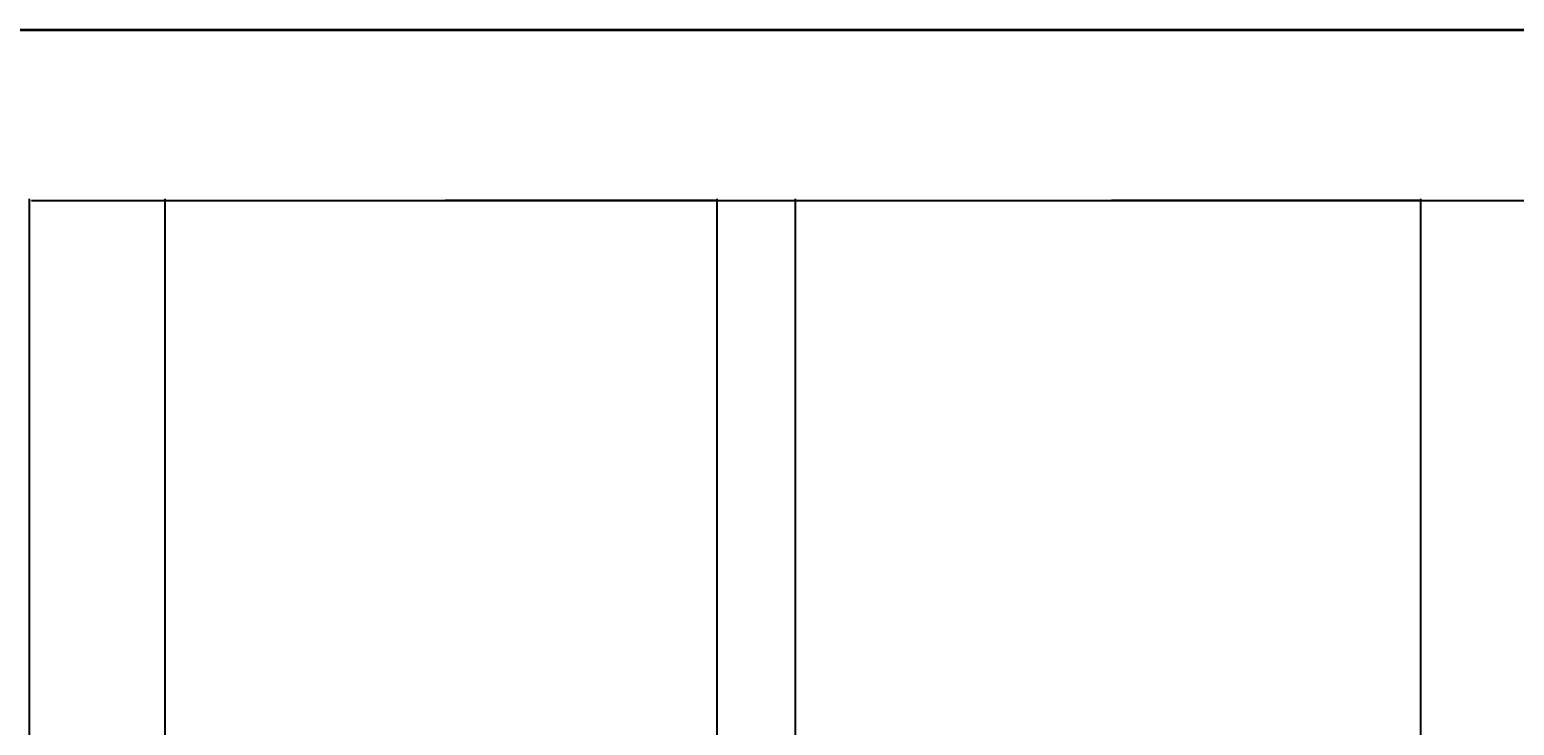
# Model space of a CAD drawing. Units: inches. Extents: x 1088 to 1703, y 668 to 1875.
# Tile 18 of 45: x 1170 to 1319, y 1805 to 1875. Entities that reach past the tile are written whole.
import ezdxf

# ---------------------------------------------------------------- set-up
doc = ezdxf.new("R2010")
doc.units = ezdxf.units.IN
doc.layers.add('A-ANNO-DIMS', color=2, linetype='Continuous', lineweight=18)
doc.layers.add('A-ANNO-TTLB', color=7, linetype='Continuous', lineweight=35)
doc.styles.get("Standard").update_dxf_attribs({"font": 'arial.ttf'})
doc.dimstyles.get("Standard").update_dxf_attribs({"dimtxt": 0.18, "dimasz": 0.18, "dimexe": 0.18, "dimexo": 0.0625, "dimgap": 0.09, "dimtad": 0, "dimtih": 1, "dimtoh": 1, "dimdec": 4, "dimzin": 0, "dimdsep": 46, "dimtxsty": 'Standard', "dimcen": 0.09, "dimadec": 0, "dimazin": 0, "dimtfac": 1, "dimtdec": 4, "dimtofl": 0, "dimtmove": 0, "dimatfit": 3, "dimfxl": 1, "dimtolj": 1, "dimtzin": 0, "dimarcsym": 0})

# ---------------------------------------------------------------- blocks, each defined once
blk = doc.blocks.new('*D28')
at = {"layer": 'A-ANNO-DIMS', "color": 0, "lineweight": -2, "transparency": 16777216}
for p, q in [((1170.34, 1803.62), (1170.34, 1857.79)), ((1170.52, 1857.61), (1408.15, 1857.61)), ((1646.56, 1857.61), (1408.94, 1857.61)), ((1646.74, 1745.55), (1646.74, 1857.79))]:
    blk.add_line(p, q, dxfattribs=at)
at = {"layer": 'A-ANNO-DIMS', "color": 0, "transparency": 16777216}
for points in [[(1170.52, 1857.64), (1170.52, 1857.58), (1170.34, 1857.61)], [(1646.56, 1857.64), (1646.56, 1857.58), (1646.74, 1857.61)]]:
    blk.add_solid(points, dxfattribs=at)
at = {"layer": 'Defpoints', "color": 0, "transparency": 16777216}
for p in [(1646.74, 1857.61), (1170.34, 1803.56), (1646.74, 1745.49)]:
    blk.add_point(p, dxfattribs=at)
at = {"layer": 'A-ANNO-DIMS', "color": 0, "transparency": 16777216, "insert": (1408.54, 1857.61), "char_height": 0.18, "attachment_point": 5}
blk.add_mtext('\\A1;476.4', dxfattribs=at)
blk = doc.blocks.new('*D35')
at = {"layer": 'A-ANNO-DIMS', "color": 0, "lineweight": -2, "transparency": 16777216}
for p, q in [((1183.89, 1448.1), (1183.89, 1857.79)), ((1184.07, 1857.61), (1211.07, 1857.61)), ((1238.86, 1857.61), (1211.86, 1857.61)), ((1239.04, 1448.1), (1239.04, 1857.79))]:
    blk.add_line(p, q, dxfattribs=at)
at = {"layer": 'A-ANNO-DIMS', "color": 0, "transparency": 16777216}
for points in [[(1184.07, 1857.64), (1184.07, 1857.58), (1183.89, 1857.61)], [(1238.86, 1857.64), (1238.86, 1857.58), (1239.04, 1857.61)]]:
    blk.add_solid(points, dxfattribs=at)
at = {"layer": 'Defpoints', "color": 0, "transparency": 16777216}
for p in [(1239.04, 1857.61), (1183.89, 1448.04), (1239.04, 1448.04)]:
    blk.add_point(p, dxfattribs=at)
at = {"layer": 'A-ANNO-DIMS', "color": 0, "transparency": 16777216, "insert": (1211.47, 1857.61), "char_height": 0.18, "attachment_point": 5}
blk.add_mtext('\\A1;55.15', dxfattribs=at)
blk = doc.blocks.new('*D36')
at = {"layer": 'A-ANNO-DIMS', "color": 0, "lineweight": -2, "transparency": 16777216}
for p, q in [((1246.85, 1448.35), (1246.85, 1857.79)), ((1247.03, 1857.61), (1277.78, 1857.61)), ((1309.17, 1857.61), (1278.43, 1857.61)), ((1309.35, 1448.35), (1309.35, 1857.79))]:
    blk.add_line(p, q, dxfattribs=at)
at = {"layer": 'A-ANNO-DIMS', "color": 0, "transparency": 16777216}
for points in [[(1247.03, 1857.64), (1247.03, 1857.58), (1246.85, 1857.61)], [(1309.17, 1857.64), (1309.17, 1857.58), (1309.35, 1857.61)]]:
    blk.add_solid(points, dxfattribs=at)
at = {"layer": 'Defpoints', "color": 0, "transparency": 16777216}
for p in [(1309.35, 1857.61), (1246.85, 1448.29), (1309.35, 1448.29)]:
    blk.add_point(p, dxfattribs=at)
at = {"layer": 'A-ANNO-DIMS', "color": 0, "transparency": 16777216, "insert": (1278.1, 1857.61), "char_height": 0.18, "attachment_point": 5}
blk.add_mtext('\\A1;62.5', dxfattribs=at)

msp = doc.modelspace()

# ---------------------------------------------------------------- linework, layer by layer
at = {"layer": 'A-ANNO-TTLB'}
msp.add_lwpolyline([(1088.369, 1874.677), (1703.181, 1874.677), (1703.181, 667.947), (1088.369, 667.947)], close=True, dxfattribs=at)

# ---------------------------------------------------------------- dimensions: what is measured, and where the dimension line sits
at = {"layer": 'A-ANNO-DIMS'}
for base, p1, p2, override, picture, middle in [((1646.743, 1857.608), (1170.345, 1803.558), (1646.743, 1745.49), {"dimdec": 1, "dimlfac": 1, "dimrnd": 0, "dimzin": 0, "dimdsep": 46, "dimlunit": 2}, '*D28', (1408.544, 1857.608)), ((1239.039, 1857.608), (1183.893, 1448.04), (1239.039, 1448.04), {"dimdec": 2, "dimlfac": 1, "dimrnd": 0, "dimzin": 0, "dimdsep": 46, "dimlunit": 2}, '*D35', (1211.466, 1857.608)), ((1309.352, 1857.608), (1246.852, 1448.287), (1309.352, 1448.287), {"dimdec": 1, "dimlfac": 1, "dimrnd": 0, "dimzin": 0, "dimdsep": 46, "dimlunit": 2}, '*D36', (1278.102, 1857.608))]:
    dim = msp.add_linear_dim(base=base, p1=p1, p2=p2, dimstyle='Standard', override=override, dxfattribs=at)
    dim.commit()
    dim.dimension.update_dxf_attribs({"geometry": picture, "text_midpoint": middle})

doc.saveas('drawing.dxf')
